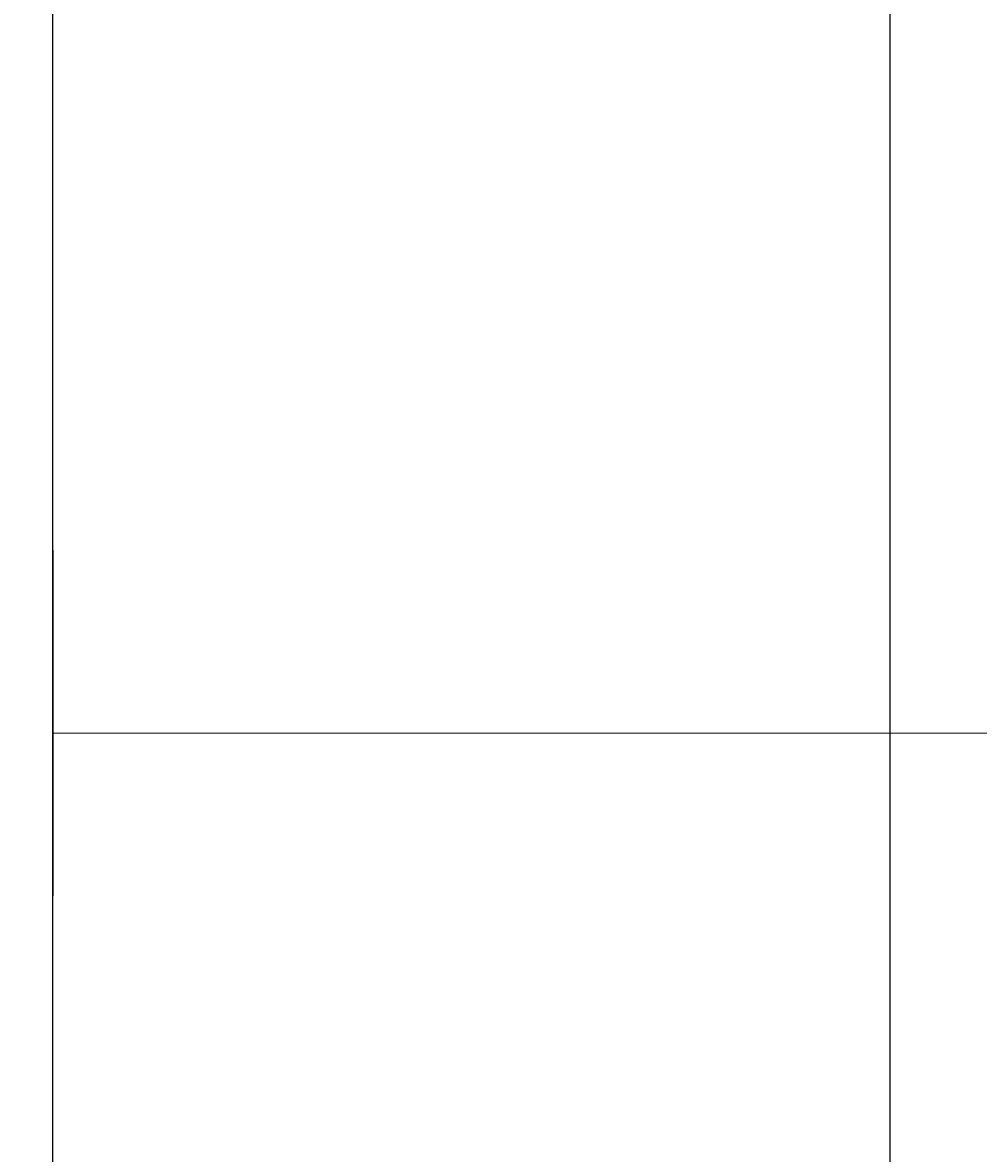
# Model space of a CAD drawing. Units: inches. Extents: x 738 to 1068, y 378 to 757.
# Tile 22 of 41: x 809 to 833, y 521 to 549. Entities that reach past the tile are written whole.
import ezdxf

# ---------------------------------------------------------------- set-up
doc = ezdxf.new("R2010")
doc.units = ezdxf.units.IN
doc.header["$MEASUREMENT"] = 0
for name, color, linetype, lineweight in [('A-ANNO-DIMS', 2, 'Continuous', 18), ('E-CTRL-CONT', 4, 'Continuous', 25), ('E-CTRL-WIRE', 7, 'Continuous', 18)]:
    doc.layers.add(name, color=color, linetype=linetype, lineweight=lineweight)
doc.styles.get("Standard").update_dxf_attribs({"font": 'arial.ttf'})
doc.dimstyles.get("Standard").update_dxf_attribs({"dimtxt": 0.18, "dimasz": 0.18, "dimexe": 0.18, "dimexo": 0.0625, "dimgap": 0.09, "dimtad": 0, "dimtih": 1, "dimtoh": 1, "dimdec": 4, "dimzin": 0, "dimdsep": 46, "dimtxsty": 'Standard', "dimcen": 0.09, "dimadec": 0, "dimazin": 0, "dimtfac": 1, "dimtdec": 4, "dimtofl": 0, "dimtmove": 0, "dimatfit": 3, "dimfxl": 1, "dimtolj": 1, "dimtzin": 0, "dimarcsym": 0})

# ---------------------------------------------------------------- blocks, each defined once
blk = doc.blocks.new('CR-AUX-CONTACT-NO')
for p, q in [((0, 8.72), (0, 0)), ((8.265, 8.72), (8.265, 0))]:
    blk.add_line(p, q)
blk = doc.blocks.new('*D32')
at = {"layer": 'A-ANNO-DIMS', "color": 0, "lineweight": -2, "transparency": 16777216}
for p, q in [((809.38, 461.454), (809.38, 756.505)), ((836.232, 461.277), (836.232, 756.505)), ((809.56, 756.325), (822.41, 756.325)), ((836.052, 756.325), (823.202, 756.325))]:
    blk.add_line(p, q, dxfattribs=at)
at = {"layer": 'A-ANNO-DIMS', "color": 0, "transparency": 16777216}
for points in [[(809.56, 756.355), (809.56, 756.295), (809.38, 756.325)], [(836.052, 756.355), (836.052, 756.295), (836.232, 756.325)]]:
    blk.add_solid(points, dxfattribs=at)
at = {"layer": 'Defpoints', "color": 0, "transparency": 16777216}
for p in [(836.232, 756.325), (809.38, 461.392), (836.232, 461.214)]:
    blk.add_point(p, dxfattribs=at)
at = {"layer": 'A-ANNO-DIMS', "color": 0, "transparency": 16777216, "insert": (822.806, 756.325), "char_height": 0.18, "attachment_point": 5}
blk.add_mtext('\\A1;26.85', dxfattribs=at)
blk = doc.blocks.new('*D34')
at = {"layer": 'A-ANNO-DIMS', "color": 0, "lineweight": -2, "transparency": 16777216}
for p, q in [((781.49, 686.266), (781.49, 378.239)), ((830.489, 686.266), (830.489, 378.239)), ((781.67, 378.419), (805.767, 378.419)), ((830.309, 378.419), (806.212, 378.419))]:
    blk.add_line(p, q, dxfattribs=at)
at = {"layer": 'A-ANNO-DIMS', "color": 0, "transparency": 16777216}
for points in [[(781.67, 378.449), (781.67, 378.389), (781.49, 378.419)], [(830.309, 378.449), (830.309, 378.389), (830.489, 378.419)]]:
    blk.add_solid(points, dxfattribs=at)
at = {"layer": 'Defpoints', "color": 0, "transparency": 16777216}
for p in [(781.49, 686.329), (830.489, 686.329), (830.489, 378.419)]:
    blk.add_point(p, dxfattribs=at)
at = {"layer": 'A-ANNO-DIMS', "color": 0, "transparency": 16777216, "insert": (805.99, 378.419), "char_height": 0.18, "attachment_point": 5}
blk.add_mtext('\\A1;49', dxfattribs=at)
blk = doc.blocks.new('*D38')
at = {"layer": 'A-ANNO-DIMS', "color": 0, "lineweight": -2, "transparency": 16777216}
for p, q in [((781.485, 593.017), (781.485, 378.239)), ((887.04, 593.067), (887.04, 378.239)), ((781.665, 378.419), (833.807, 378.419)), ((886.86, 378.419), (834.718, 378.419))]:
    blk.add_line(p, q, dxfattribs=at)
at = {"layer": 'A-ANNO-DIMS', "color": 0, "transparency": 16777216}
for points in [[(781.665, 378.449), (781.665, 378.389), (781.485, 378.419)], [(886.86, 378.449), (886.86, 378.389), (887.04, 378.419)]]:
    blk.add_solid(points, dxfattribs=at)
at = {"layer": 'Defpoints', "color": 0, "transparency": 16777216}
for p in [(781.485, 593.08), (887.04, 593.13), (887.04, 378.419)]:
    blk.add_point(p, dxfattribs=at)
at = {"layer": 'A-ANNO-DIMS', "color": 0, "transparency": 16777216, "insert": (834.263, 378.419), "char_height": 0.18, "attachment_point": 5}
blk.add_mtext('\\A1;105.56', dxfattribs=at)

msp = doc.modelspace()

# ---------------------------------------------------------------- linework, layer by layer
at = {"layer": 'E-CTRL-WIRE'}
msp.add_line((809.3803, 531.4009), (865.0964, 531.4009), dxfattribs=at)

# ---------------------------------------------------------------- block references
at = {"layer": 'E-CTRL-CONT'}
msp.add_blockref('CR-AUX-CONTACT-NO', (801.115, 527.299), dxfattribs=at)

# ---------------------------------------------------------------- dimensions: what is measured, and where the dimension line sits
at = {"layer": 'A-ANNO-DIMS'}
for base, p1, p2, override, picture, middle in [((836.2324, 756.3251), (809.3803, 461.3919), (836.2324, 461.214), {"dimdec": 2, "dimlfac": 1, "dimrnd": 0, "dimzin": 0, "dimdsep": 46, "dimlunit": 2}, '*D32', (822.8064, 756.3251)), ((830.4893, 378.4191), (781.4897, 686.329), (830.4893, 686.329), {"dimdec": 0, "dimlfac": 1, "dimrnd": 0, "dimzin": 0, "dimdsep": 46, "dimlunit": 2}, '*D34', (805.9895, 378.4191)), ((887.0404, 378.4191), (781.4846, 593.0796), (887.0404, 593.1296), {"dimdec": 2, "dimlfac": 1, "dimrnd": 0, "dimzin": 0, "dimdsep": 46, "dimlunit": 2}, '*D38', (834.2625, 378.4191))]:
    dim = msp.add_linear_dim(base=base, p1=p1, p2=p2, dimstyle='Standard', override=override, dxfattribs=at)
    dim.commit()
    dim.dimension.update_dxf_attribs({"geometry": picture, "text_midpoint": middle})

doc.saveas('drawing.dxf')
